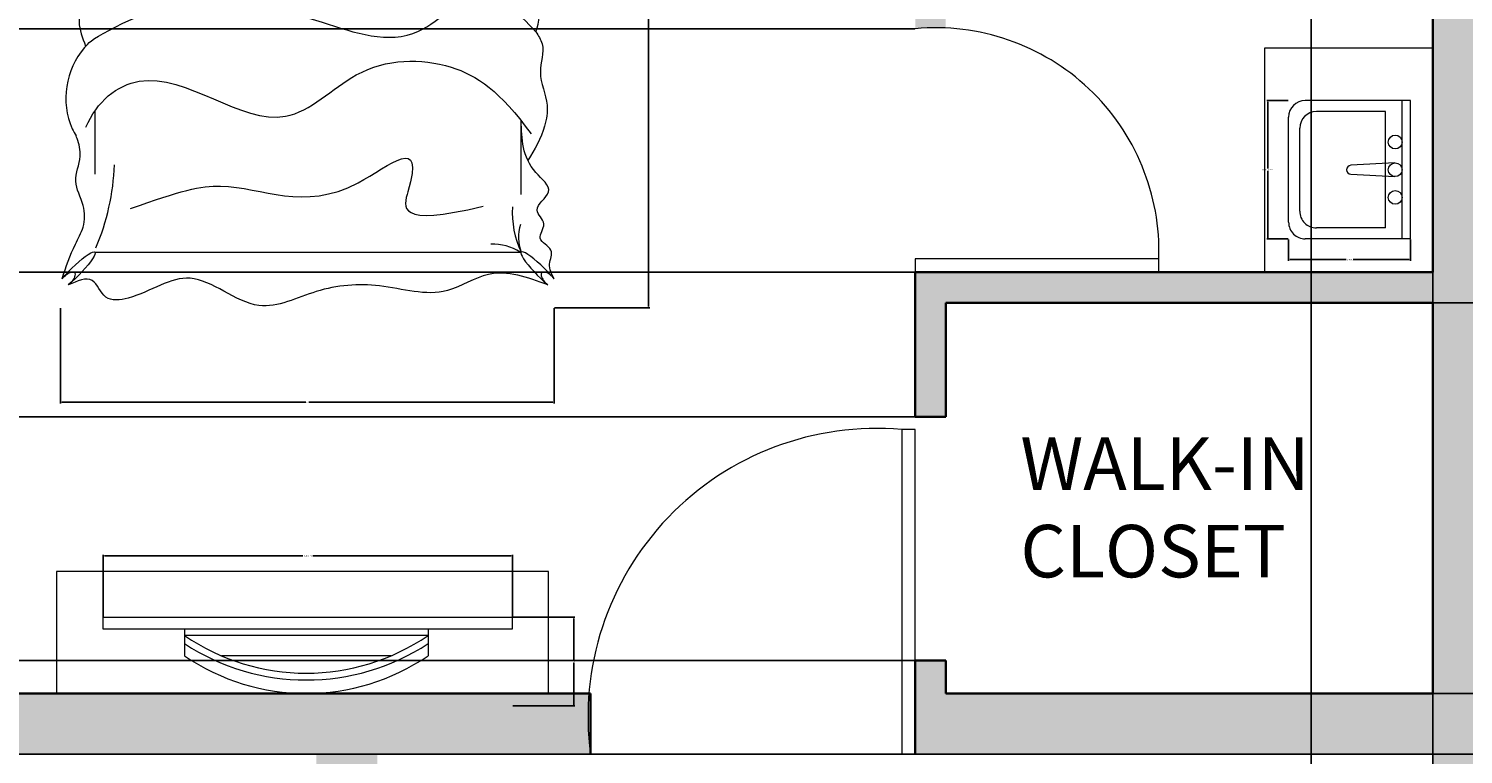
# Model space of a CAD drawing. Units: inches. Extents: x 2847 to 3693, y 1516 to 2098.
# Tile 3 of 6: x 3047 to 3259, y 1837 to 1944. Entities that reach past the tile are written whole.
import ezdxf

# ---------------------------------------------------------------- set-up
doc = ezdxf.new("R2010")
doc.units = ezdxf.units.IN
for name, color, linetype, lineweight in [('A-ANNO-DIMS', 2, 'Continuous', 18), ('A-AREA-IDEN', 7, 'Continuous', 18), ('A-DOOR', 3, 'Continuous', 18), ('A-EQPM', 9, 'Continuous', 18), ('A-FLOR-CASE', 8, 'Continuous', 18), ('A-FLOR-FIXT', 9, 'Continuous', 18), ('A-FURN', 8, 'Continuous', 18), ('A-WALL', 7, 'Continuous', 35), ('www.cadblocksfree.com', 7, 'Continuous', 9)]:
    doc.layers.add(name, color=color, linetype=linetype, lineweight=lineweight)
doc.layers.add('A-WALL-PATT', color=251, linetype='Continuous', lineweight=13, true_color=0x636466)
doc.styles.get("Standard").update_dxf_attribs({"font": 'arial.ttf'})
doc.dimstyles.get("Standard").update_dxf_attribs({"dimtxt": 0.18, "dimasz": 0.18, "dimexe": 0.18, "dimexo": 0.0625, "dimgap": 0.09, "dimtad": 0, "dimtih": 1, "dimtoh": 1, "dimdec": 4, "dimzin": 0, "dimdsep": 46, "dimtxsty": 'Standard', "dimcen": 0.09, "dimadec": 0, "dimazin": 0, "dimtfac": 1, "dimtdec": 4, "dimtofl": 0, "dimtmove": 0, "dimatfit": 3, "dimfxl": 1, "dimtolj": 1, "dimtzin": 0, "dimarcsym": 0})

# ---------------------------------------------------------------- blocks, each defined once
blk = doc.blocks.new('bed')
at = {"layer": 'www.cadblocksfree.com', "ltscale": 0.2}
h = blk.add_hatch(dxfattribs=at)
h.set_pattern_fill('ANSI37,_O', color=256, scale=0.393701)
h.set_pattern_definition([(45, (2420.7222, -262.9689), (-0.8838835, 0.8838835), []), (135, (2420.7222, -262.9689), (-0.8838835, -0.8838835), [])])
h.paths.add_polyline_path([(3417.57, 1472.4), (3372.19, 1472.4), (3372.19, 1470.94), (3417.57, 1470.94)])
for p, q in [((3363, 1473.59), (3363, 1476.25)), ((3426.76, 1473.59), (3426.76, 1476.25)), ((3372.19, 1472.4), (3417.57, 1472.4)), ((3372.19, 1470.94), (3372.19, 1472.4)), ((3417.57, 1470.94), (3417.57, 1472.4)), ((3363.39, 1470.15), (3360.88, 1467.22)), ((3372.19, 1470.94), (3417.57, 1470.94)), ((3426.38, 1470.15), (3428.88, 1467.22)), ((3409.94, 1443.85), (3408.41, 1442.96)), ((3363.39, 1412.3), (3363.39, 1402.94)), ((3426.38, 1399.91), (3426.38, 1410.81)), ((3363.39, 1391.41), (3426.38, 1391.41))]:
    blk.add_line(p, q, dxfattribs=at)
for points in [[(3426.76, 1476.25), (3363, 1476.25)], [(3361.42, 1473.89), (3361.42, 1471.52), (3372.19, 1471.52)], [(3417.57, 1471.52), (3428.35, 1471.52), (3428.35, 1473.89)], [(3426.38, 1449.41), (3426.38, 1470.15), (3363.39, 1470.15), (3363.39, 1447.08)], [(3363.39, 1445.54), (3363.39, 1443.89)], [(3363.39, 1442.49), (3363.39, 1440.37)], [(3363.39, 1438.56), (3363.39, 1431.14)]]:
    blk.add_lwpolyline(points, dxfattribs=at)
for centre, radius, start, end in [((3359.33, 1477), 3.74, 303.8271, 348.4775), ((3430.43, 1477), 3.74, 191.5225, 236.1729), ((3359.84, 1474.37), 3.25, 298.9176, 345.9939), ((3394.88, 2431.36), 958.3, 268.09356, 271.90644), ((3429.92, 1474.37), 3.25, 194.0061, 241.0824), ((3367.9, 1467.4), 1.87, 165.5166, 244.2099), ((3366.56, 1466.05), 1.87, 25.7901, 104.4834), ((3379.01, 1409.19), 58.68, 79.4235, 100.5765), ((3391.47, 1466.05), 1.87, 75.5166, 154.2099), ((3390.12, 1467.4), 1.87, 295.7901, 14.4834), ((3399.64, 1467.4), 1.87, 165.5166, 244.2099), ((3398.3, 1466.05), 1.87, 25.7901, 104.4834), ((3410.75, 1409.19), 58.68, 79.4235, 100.5765), ((3423.21, 1466.05), 1.87, 75.5166, 154.2099), ((3421.86, 1467.4), 1.87, 295.7901, 14.4834), ((3385.29, 1459.55), 19.22, 161.2852, 198.7148), ((3372.74, 1459.55), 19.22, 341.2852, 18.7148), ((3417.03, 1459.55), 19.22, 161.2852, 198.7148), ((3404.48, 1459.55), 19.22, 341.2852, 18.7148), ((3355.42, 1459.55), 13.34, 341.1598, 18.8402), ((3402.61, 1459.55), 13.34, 161.1598, 198.8402), ((3387.15, 1459.55), 13.34, 341.1598, 18.8402), ((3434.35, 1459.55), 13.34, 161.1598, 198.8402), ((3367.9, 1451.7), 1.87, 115.7901, 194.4834), ((3390.12, 1451.7), 1.87, 345.5166, 64.2099), ((3399.64, 1451.7), 1.87, 115.7901, 194.4834), ((3421.86, 1451.7), 1.87, 345.5166, 64.2099), ((3366.56, 1453.04), 1.87, 255.5166, 334.2099), ((3379.01, 1509.91), 58.68, 259.4235, 280.5765), ((3391.47, 1453.04), 1.87, 205.7901, 284.4834), ((3398.3, 1453.04), 1.87, 255.5166, 334.2099), ((3410.75, 1509.91), 58.68, 259.4235, 280.5765), ((3423.21, 1453.04), 1.87, 205.7901, 284.4834), ((3424.34, 1446.05), 3.94, 342.0511, 87.9851), ((3445.78, 1439.1), 18.6, 162.0511, 198.5657), ((3416.57, 1428.08), 12.65, 341.0268, 23.7782), ((3365.21, 1427.6), 3.94, 125.4209, 169.6982), ((3370.55, 1414.19), 11.47, 139.4648, 203.3712), ((3367.28, 1412.87), 7.94, 204.0179, 212.619), ((3331.91, 1405.56), 34.38, 336.8495, 357.9003), ((3438.82, 1397.31), 13.77, 176.7525, 205.373), ((3432.14, 1393.64), 6.17, 162.6475, 201.1361), ((3422.11, 1384.8), 7.8, 58.0013, 91.6551)]:
    blk.add_arc(centre, radius, start, end, dxfattribs=at)
at = {"layer": 'www.cadblocksfree.com', "ltscale": 0.2, "extrusion": (0, 0, -1)}
for centre, major_axis, ratio, start_param, end_param in [((3360.34, 1388.37), (3.04, 3.04), 0.168252, 4.250342, 8.316029), ((3359.29, 1387.32), (1.05, 1.05), 0.453532, 4.422107, 8.144264)]:
    blk.add_ellipse(centre, major_axis=major_axis, ratio=ratio, start_param=start_param, end_param=end_param, dxfattribs=at)
at = {"layer": 'www.cadblocksfree.com', "ltscale": 0.2}
for centre, major_axis, ratio, start_param, end_param in [((3429.42, 1388.37), (-3.04, 3.04), 0.168252, 4.250342, 8.316029), ((3430.48, 1387.32), (-1.05, 1.05), 0.453532, 4.422107, 8.144264)]:
    blk.add_ellipse(centre, major_axis=major_axis, ratio=ratio, start_param=start_param, end_param=end_param, dxfattribs=at)
for points, knots in [([(3360.88, 1467.22), (3361.27, 1466.08), (3362.33, 1462.98), (3360.73, 1458.15), (3362.39, 1452.62), (3360.35, 1448.14), (3362.43, 1444.24), (3360.04, 1441.93), (3360.26, 1438.68), (3362.05, 1436.55), (3362.42, 1434.52), (3362.57, 1432.76), (3363.1, 1431.71), (3363.39, 1431.14)], [0, 0, 0, 0, 3.550403, 9.643115, 14.356056, 20.206026, 23.427697, 25.46537, 29.172767, 31.884544, 33.668442, 35.237641, 37.145618, 37.145618, 37.145618, 37.145618]), ([(3428.88, 1467.22), (3428.49, 1466.08), (3427.44, 1462.98), (3429.04, 1458.15), (3427.38, 1452.62), (3429.08, 1448.87), (3428.37, 1446.52), (3428.27, 1446.19)], [0, 0, 0, 0, 0.0901802, 0.2449351, 0.3646438, 0.5132331, 0.5378548, 0.5378548, 0.5378548, 0.5378548]), ([(3369.63, 1465.08), (3371.1, 1465.04), (3373.63, 1464.97), (3375.26, 1462.52), (3376.48, 1462.17), (3376.75, 1462.09)], [0, 0, 0, 0, 4.163459, 7.093919, 7.934624, 7.934624, 7.934624, 7.934624]), ([(3388.54, 1465.74), (3386.72, 1465.16), (3384.36, 1464.41), (3382.68, 1461.63), (3381.45, 1461.64), (3380.81, 1461.64)], [0, 0, 0, 0, 5.530688, 7.154877, 8.940839, 8.940839, 8.940839, 8.940839]), ([(3401.22, 1465.74), (3403.05, 1465.16), (3405.41, 1464.41), (3407.09, 1461.63), (3408.31, 1461.64), (3408.95, 1461.64)], [0, 0, 0, 0, 5.530688, 7.154877, 8.940839, 8.940839, 8.940839, 8.940839]), ([(3420.14, 1465.08), (3418.66, 1465.04), (3416.14, 1464.97), (3414.5, 1462.52), (3413.28, 1462.17), (3413.01, 1462.09)], [0, 0, 0, 0, 4.163459, 7.093919, 7.934624, 7.934624, 7.934624, 7.934624]), ([(3388.36, 1460.93), (3387.64, 1460.85), (3386.25, 1460.69), (3384.48, 1459.22), (3382.96, 1459.13), (3382.11, 1459.07)], [0, 0, 0, 0, 2.127543, 4.10272, 6.58647, 6.58647, 6.58647, 6.58647]), ([(3401.41, 1460.93), (3402.13, 1460.85), (3403.51, 1460.69), (3405.28, 1459.22), (3406.81, 1459.13), (3407.65, 1459.07)], [0, 0, 0, 0, 2.127543, 4.10272, 6.58647, 6.58647, 6.58647, 6.58647]), ([(3370.05, 1456.77), (3370.59, 1457.46), (3371.71, 1458.88), (3374.68, 1457.89), (3376.51, 1458.59), (3377.52, 1458.99)], [0, 0, 0, 0, 2.388143, 4.935423, 8.166198, 8.166198, 8.166198, 8.166198]), ([(3419.72, 1456.77), (3419.17, 1457.46), (3418.05, 1458.88), (3415.08, 1457.89), (3413.26, 1458.59), (3412.24, 1458.99)], [0, 0, 0, 0, 2.388143, 4.935423, 8.166198, 8.166198, 8.166198, 8.166198]), ([(3369.29, 1453.58), (3371, 1453.6), (3374.59, 1453.64), (3377.5, 1455.76), (3379.02, 1456.87)], [0, 0, 0, 0, 5.002087, 10.507046, 10.507046, 10.507046, 10.507046]), ([(3388.77, 1454), (3388.07, 1454.76), (3386.27, 1456.73), (3383.54, 1456.81), (3381.88, 1456.86)], [0, 0, 0, 0, 3.013696, 7.735839, 7.735839, 7.735839, 7.735839]), ([(3401, 1454), (3401.7, 1454.76), (3403.5, 1456.73), (3406.22, 1456.81), (3407.88, 1456.86)], [0, 0, 0, 0, 3.013696, 7.735839, 7.735839, 7.735839, 7.735839]), ([(3420.48, 1453.58), (3418.77, 1453.6), (3415.18, 1453.64), (3412.27, 1455.76), (3410.74, 1456.87)], [0, 0, 0, 0, 5.002087, 10.507046, 10.507046, 10.507046, 10.507046]), ([(3367.27, 1444.2), (3369.57, 1444.23), (3373.92, 1444.28), (3385.47, 1449.8), (3379.56, 1446.49), (3376.81, 1444.48), (3372.95, 1444.92), (3370.93, 1443.14), (3368.77, 1443.7), (3367.36, 1443.75), (3366.55, 1443.78)], [0, 0, 0, 0, 8.61026, 16.221274, 18.843057, 23.804898, 27.440828, 29.356102, 31.203478, 33.650687, 33.650687, 33.650687, 33.650687]), ([(3409.94, 1443.85), (3413.12, 1445.84), (3417.43, 1449.66), (3422.72, 1450.04), (3424.48, 1449.98)], [1.3582378, 1.3582378, 1.3582378, 1.3582378, 1.6381418, 1.7706953, 1.7706953, 1.7706953, 1.7706953]), ([(3363.39, 1447.08), (3363.43, 1446.99), (3363.53, 1446.78), (3363.73, 1446.46), (3363.51, 1446.15), (3363.66, 1445.9), (3363.56, 1445.67), (3363.44, 1445.58), (3363.39, 1445.54)], [0, 0, 0, 0, 0.293454, 0.701471, 1.003873, 1.254893, 1.47342, 1.69185, 1.69185, 1.69185, 1.69185]), ([(3363.39, 1447.08), (3363.99, 1446.78), (3365.08, 1446.12), (3365.12, 1444.37), (3367.13, 1444.19), (3367.27, 1444.2)], [0.0122268, 0.0122268, 0.0122268, 0.0122268, 0.0594721, 0.1062177, 0.134458, 0.134458, 0.134458, 0.134458]), ([(3409.94, 1443.85), (3408.47, 1444.45), (3404.44, 1446.04), (3391.4, 1447.6), (3398.64, 1445.77), (3402.97, 1445.76), (3406.22, 1444.09), (3408.41, 1442.96)], [0.0056315, 0.0056315, 0.0056315, 0.0056315, 0.1489731, 0.3882761, 0.4793617, 0.5593494, 0.7397317, 0.7397317, 0.7397317, 0.7397317]), ([(3412.4, 1445.5), (3411.61, 1445.7), (3406.24, 1446.93), (3398.17, 1447.93), (3405.4, 1446.46), (3408.57, 1446.19), (3410.63, 1445.46), (3411.68, 1445)], [0.1043639, 0.1043639, 0.1043639, 0.1043639, 0.1489731, 0.3882761, 0.4793617, 0.5593494, 0.6446217, 0.6446217, 0.6446217, 0.6446217]), ([(3363.39, 1443.89), (3363.33, 1443.81), (3363.17, 1443.56), (3363.35, 1443.12), (3363.23, 1442.79), (3363.23, 1442.53), (3363.34, 1442.51), (3363.39, 1442.49)], [0, 0, 0, 0, 0.27176, 0.887321, 1.189132, 1.388142, 1.515331, 1.515331, 1.515331, 1.515331]), ([(3366.55, 1443.78), (3366.17, 1443.78), (3365.17, 1443.9), (3364.4, 1444.96), (3363.63, 1445.46), (3363.39, 1445.54)], [0.15648839, 0.15648839, 0.15648839, 0.15648839, 0.18439755, 0.23137648, 0.25059846, 0.25059846, 0.25059846, 0.25059846]), ([(3363.39, 1443.89), (3363.63, 1443.61), (3364.67, 1442.73), (3364.89, 1442.15), (3369.07, 1442.74), (3366.77, 1442.24), (3365.83, 1442.3), (3364.61, 1441.55), (3363.96, 1442.54), (3363.54, 1442.52), (3363.39, 1442.49)], [0.0595743, 0.0595743, 0.0595743, 0.0595743, 0.0807529, 0.1037415, 0.1697201, 0.1760361, 0.2071372, 0.2404744, 0.2623409, 0.2736605, 0.2736605, 0.2736605, 0.2736605]), ([(3362.93, 1430.81), (3365.94, 1432.96), (3375.45, 1438.99), (3392.12, 1438.03), (3404.25, 1440.73), (3408.41, 1442.96)], [0.102872, 0.102872, 0.102872, 0.102872, 0.37972, 0.957702, 1.313793, 1.313793, 1.313793, 1.313793]), ([(3363.39, 1440.37), (3363.63, 1440.51), (3364.53, 1440.9), (3366.48, 1440.25), (3370.2, 1442.29), (3367.73, 1440.64), (3365.42, 1440.07), (3364.04, 1439.91), (3363.8, 1438.94), (3363.48, 1438.64), (3363.39, 1438.56)], [0.013856, 0.013856, 0.013856, 0.013856, 0.0348738, 0.0888667, 0.1078792, 0.1267378, 0.158714, 0.1937575, 0.2174868, 0.2267221, 0.2267221, 0.2267221, 0.2267221]), ([(3363.39, 1440.37), (3363.44, 1440.27), (3363.57, 1440.06), (3363.61, 1439.68), (3363.53, 1439.31), (3363.41, 1439), (3363.33, 1438.75), (3363.37, 1438.61), (3363.39, 1438.56)], [0, 0, 0, 0, 0.329977, 0.725302, 1.129072, 1.442831, 1.734218, 1.878348, 1.878348, 1.878348, 1.878348]), ([(3365.51, 1424.21), (3370.52, 1427), (3381.15, 1429.83), (3396.21, 1425.87), (3410.54, 1420.65), (3420.27, 1432.69), (3425.88, 1426.77), (3428.53, 1423.97)], [0.099185, 0.099185, 0.099185, 0.099185, 0.523647, 0.927087, 1.289918, 1.564439, 1.810555, 1.810555, 1.810555, 1.810555]), ([(3361.34, 1428.31), (3361.33, 1428.3), (3361.16, 1427.34), (3360.78, 1425.17), (3361.47, 1423.14), (3362.01, 1421.85)], [0.3128349, 0.3128349, 0.3128349, 0.3128349, 0.313751, 0.386958, 0.4759027, 0.4759027, 0.4759027, 0.4759027]), ([(3428.53, 1423.97), (3428.91, 1423.4), (3430.1, 1421.61), (3428.49, 1417.66), (3430.59, 1413.79), (3429.8, 1409.12), (3428.4, 1406.56), (3427.36, 1404.97)], [0, 0, 0, 0, 0.050513, 0.157399, 0.2842023, 0.3628173, 0.5066917, 0.5066917, 0.5066917, 0.5066917]), ([(3362.06, 1409.87), (3363.64, 1413.65), (3372.98, 1421.34), (3389.68, 1406.04), (3402.4, 1419.98), (3416.04, 1420.17), (3423.23, 1415.23), (3427.83, 1408.9)], [0.029901, 0.029901, 0.029901, 0.029901, 0.276967, 0.797115, 1.093669, 1.464666, 1.788489, 1.788489, 1.788489, 1.788489]), ([(3431.24, 1387.47), (3430.88, 1388.17), (3430.2, 1389.5), (3431.48, 1391.99), (3428.29, 1393.19), (3430.5, 1395.69), (3427.56, 1397.87), (3431.84, 1400.39), (3426.54, 1404.33), (3426.44, 1408.15), (3426.38, 1410.81)], [0, 0, 0, 0, 2.267059, 4.324559, 6.685584, 8.878641, 11.121502, 14.300359, 17.755284, 25.682856, 25.682856, 25.682856, 25.682856]), ([(3358.53, 1387.47), (3359.1, 1389.21), (3359.96, 1391.82), (3361.92, 1395.15), (3361.9, 1398.55), (3359.88, 1401.84), (3361.56, 1405.21), (3361.03, 1407.51), (3360.64, 1408.47), (3360.59, 1408.59)], [0, 0, 0, 0, 0.138875, 0.2092702, 0.2901949, 0.3858479, 0.4804923, 0.5489252, 0.5590752, 0.5590752, 0.5590752, 0.5590752]), ([(3368.63, 1397.84), (3375.98, 1400.49), (3385.35, 1402.76), (3397.53, 1395.27), (3413.59, 1410.38), (3407.81, 1395.02), (3420.76, 1398.2)], [0.029901, 0.029901, 0.029901, 0.029901, 0.276967, 0.797115, 1.093669, 1.16836, 1.16836, 1.16836, 1.16836]), ([(3430.32, 1386.56), (3427.33, 1387.65), (3422.15, 1389.55), (3414.53, 1384.14), (3405.61, 1387.05), (3396.29, 1386.31), (3386.84, 1381.28), (3377.74, 1390.27), (3370.78, 1384.8), (3364.63, 1383.97), (3363.28, 1388.27), (3360.78, 1387.15), (3359.45, 1386.56)], [0, 0, 0, 0, 8.93042, 15.449194, 25.485629, 34.878505, 43.598887, 54.554403, 64.16647, 67.461673, 70.610457, 74.213583, 74.213583, 74.213583, 74.213583])]:
    blk.add_open_spline(points, degree=3, knots=knots, dxfattribs=at)
for points in [[(3361.23, 1424.04), (3361.24, 1424.04), (3361.24, 1424.04), (3361.24, 1424.04)], [(3361.84, 1421.64), (3362.35, 1422.25), (3362.87, 1422.86), (3365.51, 1424.21)]]:
    blk.add_open_spline(points, degree=3, dxfattribs=at)
blk = doc.blocks.new('Television')
for p, q in [((2488.56, 2041.12), (2484.64, 2041.12)), ((2487.64, 2005.12), (2487.64, 2041.12)), ((2484.64, 2010.57), (2484.64, 2035.66)), ((2488.56, 2005.12), (2484.64, 2005.12))]:
    blk.add_line(p, q)
blk.add_lwpolyline([(2488.56, 2053.12), (2490.33, 2053.12), (2490.33, 1992.66), (2488.56, 1992.66)], close=True)
for centre, radius, start, end in [((2510.99, 2023.12), 31.91, 145.6614, 214.3386), ((2513.92, 2023.12), 32.85, 146.7698, 213.2302), ((2513.92, 2023.12), 31.85, 145.583, 214.417)]:
    blk.add_arc(centre, radius, start, end)
blk = doc.blocks.new('A$C5C4020F2')
for p, q in [((0.5, 0.44), (0, 0.44)), ((0, 0.44), (0, 0.06)), ((0.5, 0.44), (0.5, 0.06)), ((0.5, 0.41), (0, 0.41)), ((0.225, 0.3836), (0.234, 0.2241)), ((0.266, 0.2241), (0.275, 0.3836)), ((0.04, 0.35), (0.04, 0.1)), ((0.46, 0.35), (0.04, 0.35)), ((0.46, 0.35), (0.46, 0.1)), ((0.4, 0.04), (0.1, 0.04)), ((0.44, 0), (0.06, 0))]:
    blk.add_line(p, q)
for centre in [(0.15, 0.385), (0.25, 0.385), (0.35, 0.385)]:
    blk.add_circle(centre, 0.025)
for centre, radius, start, end in [((0.25, 0.225), 0.016, 183.2169, 356.7831), ((0.06, 0.06), 0.06, 180, 270), ((0.1, 0.1), 0.06, 180, 270), ((0.4, 0.1), 0.06, 270, 0), ((0.44, 0.06), 0.06, 270, 0)]:
    blk.add_arc(centre, radius, start, end)
blk = doc.blocks.new('*D19')
at = {"layer": 'A-ANNO-DIMS', "color": 0, "lineweight": -2, "transparency": 16777216}
for p, q in [((3233.47, 1933.75), (3230.29, 1933.75)), ((3230.47, 1933.57), (3230.47, 1923.71)), ((3230.47, 1913.48), (3230.47, 1923.34)), ((3233.47, 1913.3), (3230.29, 1913.3))]:
    blk.add_line(p, q, dxfattribs=at)
at = {"layer": 'A-ANNO-DIMS', "color": 0, "transparency": 16777216}
for points in [[(3230.44, 1933.57), (3230.5, 1933.57), (3230.47, 1933.75)], [(3230.44, 1913.48), (3230.5, 1913.48), (3230.47, 1913.3)]]:
    blk.add_solid(points, dxfattribs=at)
at = {"layer": 'Defpoints', "color": 0, "transparency": 16777216}
for p in [(3233.53, 1933.75), (3230.47, 1913.3), (3233.53, 1913.3)]:
    blk.add_point(p, dxfattribs=at)
at = {"layer": 'A-ANNO-DIMS', "color": 0, "transparency": 16777216, "insert": (3230.47, 1923.52), "char_height": 0.18, "attachment_point": 5}
blk.add_mtext('\\A1;BASIN 20 TYP.', dxfattribs=at)
blk = doc.blocks.new('*D20')
at = {"layer": 'A-ANNO-DIMS', "color": 0, "lineweight": -2, "transparency": 16777216}
for p, q in [((3233.53, 1913.23), (3233.53, 1910.05)), ((3251.54, 1913.23), (3251.54, 1910.05)), ((3233.71, 1910.23), (3242.02, 1910.23)), ((3251.36, 1910.23), (3243.05, 1910.23))]:
    blk.add_line(p, q, dxfattribs=at)
at = {"layer": 'A-ANNO-DIMS', "color": 0, "transparency": 16777216}
for points in [[(3233.71, 1910.26), (3233.71, 1910.2), (3233.53, 1910.23)], [(3251.36, 1910.26), (3251.36, 1910.2), (3251.54, 1910.23)]]:
    blk.add_solid(points, dxfattribs=at)
at = {"layer": 'Defpoints', "color": 0, "transparency": 16777216}
for p in [(3233.53, 1913.3), (3251.54, 1913.3), (3251.54, 1910.23)]:
    blk.add_point(p, dxfattribs=at)
at = {"layer": 'A-ANNO-DIMS', "color": 0, "transparency": 16777216, "insert": (3242.54, 1910.23), "char_height": 0.18, "attachment_point": 5}
blk.add_mtext('\\A1;18 TYP.', dxfattribs=at)
blk = doc.blocks.new('*D21')
at = {"layer": 'A-ANNO-DIMS', "color": 0, "lineweight": -2, "transparency": 16777216}
for p, q in [((3125.04, 1996.19), (3139.12, 1996.19)), ((3138.94, 1996.01), (3138.94, 1949.83)), ((3138.94, 1903.3), (3138.94, 1949.47)), ((3125.04, 1903.12), (3139.12, 1903.12))]:
    blk.add_line(p, q, dxfattribs=at)
at = {"layer": 'A-ANNO-DIMS', "color": 0, "transparency": 16777216}
for points in [[(3138.91, 1996.01), (3138.97, 1996.01), (3138.94, 1996.19)], [(3138.91, 1903.3), (3138.97, 1903.3), (3138.94, 1903.12)]]:
    blk.add_solid(points, dxfattribs=at)
at = {"layer": 'Defpoints', "color": 0, "transparency": 16777216}
for p in [(3124.97, 1996.19), (3138.94, 1996.19), (3124.97, 1903.12)]:
    blk.add_point(p, dxfattribs=at)
at = {"layer": 'A-ANNO-DIMS', "color": 0, "transparency": 16777216, "insert": (3138.94, 1949.65), "char_height": 0.18, "attachment_point": 5}
blk.add_mtext('\\A1;BED 93', dxfattribs=at)
blk = doc.blocks.new('*D22')
at = {"layer": 'A-ANNO-DIMS', "color": 0, "lineweight": -2, "transparency": 16777216}
for p, q in [((3052.03, 1903.05), (3052.03, 1888.98)), ((3124.97, 1903.05), (3124.97, 1888.98)), ((3052.21, 1889.16), (3088.28, 1889.16)), ((3124.79, 1889.16), (3088.72, 1889.16))]:
    blk.add_line(p, q, dxfattribs=at)
at = {"layer": 'A-ANNO-DIMS', "color": 0, "transparency": 16777216}
for points in [[(3052.21, 1889.19), (3052.21, 1889.13), (3052.03, 1889.16)], [(3124.79, 1889.19), (3124.79, 1889.13), (3124.97, 1889.16)]]:
    blk.add_solid(points, dxfattribs=at)
at = {"layer": 'Defpoints', "color": 0, "transparency": 16777216}
for p in [(3052.03, 1903.12), (3124.97, 1903.12), (3124.97, 1889.16)]:
    blk.add_point(p, dxfattribs=at)
at = {"layer": 'A-ANNO-DIMS', "color": 0, "transparency": 16777216, "insert": (3088.5, 1889.16), "char_height": 0.18, "attachment_point": 5}
blk.add_mtext('\\A1;73', dxfattribs=at)
blk = doc.blocks.new('*D23')
at = {"layer": 'A-ANNO-DIMS', "color": 0, "lineweight": -2, "transparency": 16777216}
for p, q in [((3058.35, 1857.43), (3058.35, 1866.62)), ((3058.53, 1866.44), (3087.83, 1866.44)), ((3118.63, 1866.44), (3089.32, 1866.44)), ((3118.81, 1857.43), (3118.81, 1866.62))]:
    blk.add_line(p, q, dxfattribs=at)
at = {"layer": 'A-ANNO-DIMS', "color": 0, "transparency": 16777216}
for points in [[(3058.53, 1866.47), (3058.53, 1866.41), (3058.35, 1866.44)], [(3118.63, 1866.47), (3118.63, 1866.41), (3118.81, 1866.44)]]:
    blk.add_solid(points, dxfattribs=at)
at = {"layer": 'Defpoints', "color": 0, "transparency": 16777216}
for p in [(3058.35, 1866.44), (3058.35, 1857.37), (3118.81, 1857.37)]:
    blk.add_point(p, dxfattribs=at)
at = {"layer": 'A-ANNO-DIMS', "color": 0, "transparency": 16777216, "insert": (3088.58, 1866.44), "char_height": 0.18, "attachment_point": 5}
blk.add_mtext('\\A1;TV UNIT 60', dxfattribs=at)
blk = doc.blocks.new('*D24')
at = {"layer": 'A-ANNO-DIMS', "color": 0, "lineweight": -2, "transparency": 16777216}
for p, q in [((3118.87, 1857.37), (3128.06, 1857.37)), ((3127.88, 1857.19), (3127.88, 1851)), ((3127.88, 1844.44), (3127.88, 1850.63)), ((3118.87, 1844.26), (3128.06, 1844.26))]:
    blk.add_line(p, q, dxfattribs=at)
at = {"layer": 'A-ANNO-DIMS', "color": 0, "transparency": 16777216}
for points in [[(3127.85, 1857.19), (3127.91, 1857.19), (3127.88, 1857.37)], [(3127.85, 1844.44), (3127.91, 1844.44), (3127.88, 1844.26)]]:
    blk.add_solid(points, dxfattribs=at)
at = {"layer": 'Defpoints', "color": 0, "transparency": 16777216}
for p in [(3118.81, 1857.37), (3127.88, 1857.37), (3118.81, 1844.26)]:
    blk.add_point(p, dxfattribs=at)
at = {"layer": 'A-ANNO-DIMS', "color": 0, "transparency": 16777216, "insert": (3127.88, 1850.82), "char_height": 0.18, "attachment_point": 5}
blk.add_mtext('\\A1;13', dxfattribs=at)
blk = doc.blocks.new('*D50')
at = {"layer": 'A-ANNO-DIMS', "color": 0, "lineweight": -2, "transparency": 16777216}
for p, q in [((2989.41, 2011.12), (3692.73, 2011.12)), ((3692.55, 2010.94), (3692.55, 1924.3)), ((3692.55, 1837.3), (3692.55, 1923.94)), ((2989.41, 1837.12), (3692.73, 1837.12))]:
    blk.add_line(p, q, dxfattribs=at)
at = {"layer": 'A-ANNO-DIMS', "color": 0, "transparency": 16777216}
for points in [[(3692.52, 2010.94), (3692.58, 2010.94), (3692.55, 2011.12)], [(3692.52, 1837.3), (3692.58, 1837.3), (3692.55, 1837.12)]]:
    blk.add_solid(points, dxfattribs=at)
at = {"layer": 'Defpoints', "color": 0, "transparency": 16777216}
for p in [(2989.35, 2011.12), (3692.55, 2011.12), (2989.35, 1837.12)]:
    blk.add_point(p, dxfattribs=at)
at = {"layer": 'A-ANNO-DIMS', "color": 0, "transparency": 16777216, "insert": (3692.55, 1924.12), "char_height": 0.18, "attachment_point": 5}
blk.add_mtext('\\A1;174', dxfattribs=at)
blk = doc.blocks.new('*D55')
at = {"layer": 'A-ANNO-DIMS', "color": 0, "lineweight": -2, "transparency": 16777216}
for p, q in [((3178.28, 1944.37), (2846.97, 1944.37)), ((2847.15, 1944.19), (2847.15, 1926.55)), ((2847.15, 1908.55), (2847.15, 1926.19)), ((3178.28, 1908.37), (2846.97, 1908.37))]:
    blk.add_line(p, q, dxfattribs=at)
at = {"layer": 'A-ANNO-DIMS', "color": 0, "transparency": 16777216}
for points in [[(2847.12, 1944.19), (2847.18, 1944.19), (2847.15, 1944.37)], [(2847.12, 1908.55), (2847.18, 1908.55), (2847.15, 1908.37)]]:
    blk.add_solid(points, dxfattribs=at)
at = {"layer": 'Defpoints', "color": 0, "transparency": 16777216}
for p in [(2847.15, 1944.37), (3178.35, 1944.37), (3178.35, 1908.37)]:
    blk.add_point(p, dxfattribs=at)
at = {"layer": 'A-ANNO-DIMS', "color": 0, "transparency": 16777216, "insert": (2847.15, 1926.37), "char_height": 0.18, "attachment_point": 5}
blk.add_mtext('\\A1;36', dxfattribs=at)
blk = doc.blocks.new('*D56')
at = {"layer": 'A-ANNO-DIMS', "color": 0, "lineweight": -2, "transparency": 16777216}
for p, q in [((3182.91, 1903.87), (3692.73, 1903.87)), ((3692.55, 1903.69), (3692.55, 1875.17)), ((3692.55, 1846.3), (3692.55, 1874.81)), ((3182.91, 1846.12), (3692.73, 1846.12))]:
    blk.add_line(p, q, dxfattribs=at)
at = {"layer": 'A-ANNO-DIMS', "color": 0, "transparency": 16777216}
for points in [[(3692.52, 1903.69), (3692.58, 1903.69), (3692.55, 1903.87)], [(3692.52, 1846.3), (3692.58, 1846.3), (3692.55, 1846.12)]]:
    blk.add_solid(points, dxfattribs=at)
at = {"layer": 'Defpoints', "color": 0, "transparency": 16777216}
for p in [(3182.85, 1903.87), (3692.55, 1903.87), (3182.85, 1846.12)]:
    blk.add_point(p, dxfattribs=at)
at = {"layer": 'A-ANNO-DIMS', "color": 0, "transparency": 16777216, "insert": (3692.55, 1874.99), "char_height": 0.18, "attachment_point": 5}
blk.add_mtext('\\A1;57.75', dxfattribs=at)
blk = doc.blocks.new('*D74')
at = {"layer": 'A-ANNO-DIMS', "color": 0, "lineweight": -2, "transparency": 16777216}
for p, q in [((3182.78, 1886.99), (2846.97, 1886.99)), ((2847.15, 1886.81), (2847.15, 1869.17)), ((2847.15, 1851.17), (2847.15, 1868.81)), ((3182.78, 1850.99), (2846.97, 1850.99))]:
    blk.add_line(p, q, dxfattribs=at)
at = {"layer": 'A-ANNO-DIMS', "color": 0, "transparency": 16777216}
for points in [[(2847.12, 1886.81), (2847.18, 1886.81), (2847.15, 1886.99)], [(2847.12, 1851.17), (2847.18, 1851.17), (2847.15, 1850.99)]]:
    blk.add_solid(points, dxfattribs=at)
at = {"layer": 'Defpoints', "color": 0, "transparency": 16777216}
for p in [(3182.85, 1886.99), (2847.15, 1850.99), (3182.85, 1850.99)]:
    blk.add_point(p, dxfattribs=at)
at = {"layer": 'A-ANNO-DIMS', "color": 0, "transparency": 16777216, "insert": (2847.15, 1868.99), "char_height": 0.18, "attachment_point": 5}
blk.add_mtext('\\A1;36', dxfattribs=at)
blk = doc.blocks.new('*D75')
at = {"layer": 'A-ANNO-DIMS', "color": 0, "lineweight": -2, "transparency": 16777216}
for p, q in [((3236.85, 2002.06), (3236.85, 1516.24)), ((3254.85, 2002.06), (3254.85, 1516.24)), ((3237.03, 1516.42), (3245.64, 1516.42)), ((3254.67, 1516.42), (3246.06, 1516.42))]:
    blk.add_line(p, q, dxfattribs=at)
at = {"layer": 'A-ANNO-DIMS', "color": 0, "transparency": 16777216}
for points in [[(3237.03, 1516.45), (3237.03, 1516.39), (3236.85, 1516.42)], [(3254.67, 1516.45), (3254.67, 1516.39), (3254.85, 1516.42)]]:
    blk.add_solid(points, dxfattribs=at)
at = {"layer": 'Defpoints', "color": 0, "transparency": 16777216}
for p in [(3236.85, 2002.12), (3254.85, 2002.12), (3254.85, 1516.42)]:
    blk.add_point(p, dxfattribs=at)
at = {"layer": 'A-ANNO-DIMS', "color": 0, "transparency": 16777216, "insert": (3245.85, 1516.42), "char_height": 0.18, "attachment_point": 5}
blk.add_mtext('\\A1;18', dxfattribs=at)

msp = doc.modelspace()

# ---------------------------------------------------------------- hatches: boundary and pattern name
at = {"layer": 'A-WALL-PATT'}
h = msp.add_hatch(color=256, dxfattribs=at)
h.dxf.hatch_style = 1
h.paths.add_polyline_path([(2998.3457, 2002.118), (3178.3457, 2002.118), (3178.3457, 1944.368, -0.0341147), (3182.8457, 1944.4698), (3182.8457, 2002.118), (3200.8457, 2002.118), (3200.8457, 2011.118), (2989.3457, 2011.118), (2989.3457, 1960.118), (2998.3457, 1960.118)])
h.paths.add_polyline_path([(2998.3457, 1888.118), (2989.3457, 1888.118), (2989.3457, 1837.118), (3089.8457, 1837.118), (3089.8457, 1778.618), (3098.8457, 1778.618), (3098.8457, 1837.118), (3130.3457, 1837.118, -0.05293254), (3130.1282, 1846.118), (2998.3457, 1846.118)])
h.paths.add_polyline_path([(3263.8457, 2002.118), (3311.8457, 2002.118), (3311.8457, 2011.118), (3263.8457, 2011.118), (3236.8457, 2011.118), (3236.8457, 2002.118), (3254.8457, 2002.118), (3254.8457, 1908.368), (3182.8457, 1908.368), (3178.3457, 1908.368), (3178.3457, 1886.993), (3182.8457, 1886.993), (3182.8457, 1903.868), (3254.8457, 1903.868), (3254.8457, 1846.118), (3182.8457, 1846.118), (3182.8457, 1850.993), (3178.3457, 1850.993), (3178.3457, 1837.118), (3254.8457, 1837.118), (3254.8457, 1790.618), (3263.8457, 1790.618), (3263.8457, 1837.118)])
h.paths.add_polyline_path([(2930.8457, 1837.118), (2921.8457, 1837.118), (2921.8457, 1828.118), (2930.8457, 1828.118)])
h.paths.add_polyline_path([(2930.8457, 1600.118), (2921.8457, 1600.118), (2921.8457, 1591.118), (2930.8457, 1591.118)])
h.paths.add_polyline_path([(3098.8457, 1658.618), (3089.8457, 1658.618), (3089.8457, 1591.118), (3140.8457, 1591.118), (3140.8457, 1600.118), (3098.8457, 1600.118)])
h.paths.add_polyline_path([(3305.8457, 1600.118), (3263.8457, 1600.118), (3263.8457, 1646.618), (3254.8457, 1646.618), (3254.8457, 1600.118), (3212.8457, 1600.118), (3212.8457, 1591.118), (3254.8457, 1591.118), (3305.8457, 1591.118)])
h.paths.add_polyline_path([(3470.8457, 1600.118), (3428.8457, 1600.118), (3428.8457, 1756.118), (3430.26, 1756.118), (3430.26, 1765.118), (3428.8457, 1765.118), (3419.8457, 1765.118), (3419.8457, 1600.118), (3377.8457, 1600.118), (3377.8457, 1591.118), (3470.8457, 1591.118)])
h.paths.add_polyline_path([(3593.8457, 1642.118), (3584.8457, 1642.118), (3584.8457, 1600.118), (3542.8457, 1600.118), (3542.8457, 1591.118), (3593.8457, 1591.118)])
h.paths.add_polyline_path([(3593.8457, 1796.083), (3584.8457, 1796.083), (3584.8457, 1765.118), (3505.3457, 1765.118), (3505.3457, 1837.118), (3584.8457, 1837.118), (3584.8457, 1832.083), (3593.8457, 1832.083), (3593.8457, 1837.118), (3593.8457, 1924.118), (3584.8457, 1924.118), (3584.8457, 1846.118), (3478.26, 1846.118), (3478.26, 1837.118), (3500.8457, 1837.118), (3500.8457, 1765.118), (3478.26, 1765.118, -0.03536449), (3478.26, 1758.7816), (3478.26, 1756.118), (3584.8457, 1756.118), (3584.8457, 1714.118), (3593.8457, 1714.118)])
h.paths.add_polyline_path([(3593.8457, 2011.118), (3536.8457, 2011.118), (3536.8457, 2002.118), (3584.8457, 2002.118), (3584.8457, 1960.118), (3593.8457, 1960.118)])
h.paths.add_polyline_path([(3476.8457, 2011.118), (3371.8457, 2011.118), (3371.8457, 2002.118), (3419.8457, 2002.118), (3419.8457, 1837.118), (3428.8457, 1837.118), (3430.26, 1837.118), (3430.26, 1846.118), (3428.8457, 1846.118), (3428.8457, 2002.118), (3476.8457, 2002.118)])

# ---------------------------------------------------------------- linework, layer by layer
at = {"layer": 'A-DOOR'}
for p, q in [((3214.3457, 1910.368), (3178.3457, 1910.368)), ((3178.3457, 1910.368), (3178.3457, 1908.368)), ((3214.3457, 1908.368), (3214.3457, 1910.368)), ((3178.3457, 1908.368), (3214.3457, 1908.368)), ((3178.3457, 1885.118), (3176.3457, 1885.118)), ((3176.3457, 1885.118), (3176.3457, 1837.118)), ((3178.3457, 1837.118), (3178.3457, 1885.118))]:
    msp.add_line(p, q, dxfattribs=at)
for centre, radius, start, end in [((3181.3406, 1911.4803), 33.0238, 358.069858, 95.203296), ((3172.6248, 1842.6422), 42.6385, 84.993649, 187.444101)]:
    msp.add_arc(centre, radius, start, end, dxfattribs=at)
at = {"layer": 'A-FLOR-CASE'}
for p, q in [((3230.0135, 1908.368), (3230.0135, 1941.5616)), ((3230.0135, 1941.5616), (3254.8457, 1941.5616)), ((3124.1443, 1864.118), (3051.4532, 1864.118)), ((3051.4532, 1864.118), (3051.4532, 1846.118)), ((3124.1443, 1846.118), (3124.1443, 1864.118))]:
    msp.add_line(p, q, dxfattribs=at)
at = {"layer": 'A-WALL'}
for p, q in [((3254.8457, 1908.368), (3254.8457, 2002.118)), ((3178.3457, 1886.993), (3178.3457, 1908.368)), ((3182.8457, 1908.368), (3178.3457, 1908.368)), ((3182.8457, 1908.368), (3254.8457, 1908.368)), ((3182.8457, 1903.868), (3254.8457, 1903.868)), ((3182.8457, 1886.993), (3182.8457, 1903.868)), ((3254.8457, 1846.118), (3254.8457, 1903.868)), ((3182.8457, 1886.993), (3178.3457, 1886.993)), ((3178.3457, 1846.118), (3178.3457, 1850.993)), ((3182.8457, 1850.993), (3178.3457, 1850.993)), ((3182.8457, 1846.118), (3182.8457, 1850.993)), ((2998.3457, 1846.118), (3130.3457, 1846.118)), ((3130.3457, 1846.118), (3130.3457, 1837.118)), ((3178.3457, 1846.118), (3178.3457, 1837.118)), ((3182.8457, 1846.118), (3254.8457, 1846.118))]:
    msp.add_line(p, q, dxfattribs=at)

# ---------------------------------------------------------------- block references
at = {"layer": 'A-EQPM', "rotation": 90}
msp.add_blockref('Television', (5111.4641, -632.9653), dxfattribs=at)
at = {"layer": 'A-FLOR-FIXT', "xscale": 40.9105995528571, "yscale": 40.9105995528571, "zscale": 40.9105995528571, "rotation": 270}
msp.add_blockref('A$C5C4020F2', (3233.5349, 1933.7521), dxfattribs=at)
at = {"layer": 'A-FURN'}
msp.add_blockref('bed', (-306.2617, 519.939), dxfattribs=at)

# ---------------------------------------------------------------- texts
at = {"layer": 'A-AREA-IDEN', "insert": (3193.8856, 1883.96), "char_height": 7.75699, "attachment_point": 1}
msp.add_mtext_dynamic_manual_height_columns('WALK-IN\\PCLOSET', width=207.07675, gutter_width=38.785, heights=[0], dxfattribs=at)

# ---------------------------------------------------------------- dimensions: what is measured, and where the dimension line sits
at = {"layer": 'A-ANNO-DIMS'}
for base, p1, p2, override, picture, middle in [((3692.5457, 2011.118), (2989.3457, 1837.118), (2989.3457, 2011.118), {"dimdec": 0, "dimlfac": 1, "dimrnd": 0, "dimzin": 0, "dimdsep": 46, "dimlunit": 2}, '*D50', (3692.5457, 1924.118)), ((2847.1457, 1944.368), (3178.3457, 1908.368), (3178.3457, 1944.368), {"dimdec": 0, "dimlfac": 1, "dimrnd": 0, "dimzin": 0, "dimdsep": 46, "dimlunit": 2}, '*D55', (2847.1457, 1926.368)), ((3692.5457, 1903.868), (3182.8457, 1846.118), (3182.8457, 1903.868), {"dimdec": 2, "dimlfac": 1, "dimrnd": 0, "dimzin": 0, "dimdsep": 46, "dimlunit": 2}, '*D56', (3692.5457, 1874.993)), ((2847.1457, 1850.993), (3182.8457, 1886.993), (3182.8457, 1850.993), {"dimdec": 0, "dimlfac": 1, "dimrnd": 0, "dimzin": 0, "dimdsep": 46, "dimlunit": 2}, '*D74', (2847.1457, 1868.993)), ((3127.8771, 1857.3664), (3118.8078, 1844.2642), (3118.8078, 1857.3664), {"dimdec": 0, "dimlfac": 1, "dimrnd": 0, "dimzin": 0, "dimdsep": 46, "dimlunit": 2}, '*D24', (3127.8771, 1850.8153))]:
    dim = msp.add_linear_dim(base=base, p1=p1, p2=p2, angle=90, dimstyle='Standard', override=override, dxfattribs=at)
    dim.commit()
    dim.dimension.update_dxf_attribs({"geometry": picture, "text_midpoint": middle})
for base, p1, p2, picture, middle in [((3254.8457, 1516.418), (3236.8457, 2002.118), (3254.8457, 2002.118), '*D75', (3245.8457, 1516.418)), ((3124.975, 1889.1566), (3052.0279, 1903.1171), (3124.975, 1903.1171), '*D22', (3088.5015, 1889.1566))]:
    dim = msp.add_linear_dim(base=base, p1=p1, p2=p2, dimstyle='Standard', override={"dimdec": 0, "dimlfac": 1, "dimrnd": 0, "dimzin": 0, "dimdsep": 46, "dimlunit": 2}, dxfattribs=at)
    dim.commit()
    dim.dimension.update_dxf_attribs({"geometry": picture, "text_midpoint": middle})
for base, p1, p2, angle, text, picture, middle in [((3138.9356, 1996.1877), (3124.975, 1903.1171), (3124.975, 1996.1877), 90, 'BED <>', '*D21', (3138.9356, 1949.6524)), ((3230.4666, 1913.2968), (3233.5349, 1933.7521), (3233.5349, 1913.2968), 270, 'BASIN <> TYP.', '*D19', (3230.4666, 1923.5244)), ((3058.3457, 1866.4357), (3118.8078, 1857.3664), (3058.3457, 1857.3664), 180, 'TV UNIT <>', '*D23', (3088.5767, 1866.4357))]:
    dim = msp.add_linear_dim(base=base, p1=p1, p2=p2, angle=angle, text=text, dimstyle='Standard', override={"dimdec": 0, "dimlfac": 1, "dimrnd": 0, "dimzin": 0, "dimdsep": 46, "dimlunit": 2}, dxfattribs=at)
    dim.commit()
    dim.dimension.update_dxf_attribs({"geometry": picture, "text_midpoint": middle})
dim = msp.add_linear_dim(base=(3251.5355, 1910.2285), p1=(3233.5349, 1913.2968), p2=(3251.5355, 1913.2968), text='<> TYP.', dimstyle='Standard', override={"dimdec": 0, "dimlfac": 1, "dimrnd": 0, "dimzin": 0, "dimdsep": 46, "dimlunit": 2}, dxfattribs=at)
dim.commit()
dim.dimension.update_dxf_attribs({"geometry": '*D20', "text_midpoint": (3242.5352, 1910.2285)})

doc.saveas('drawing.dxf')
